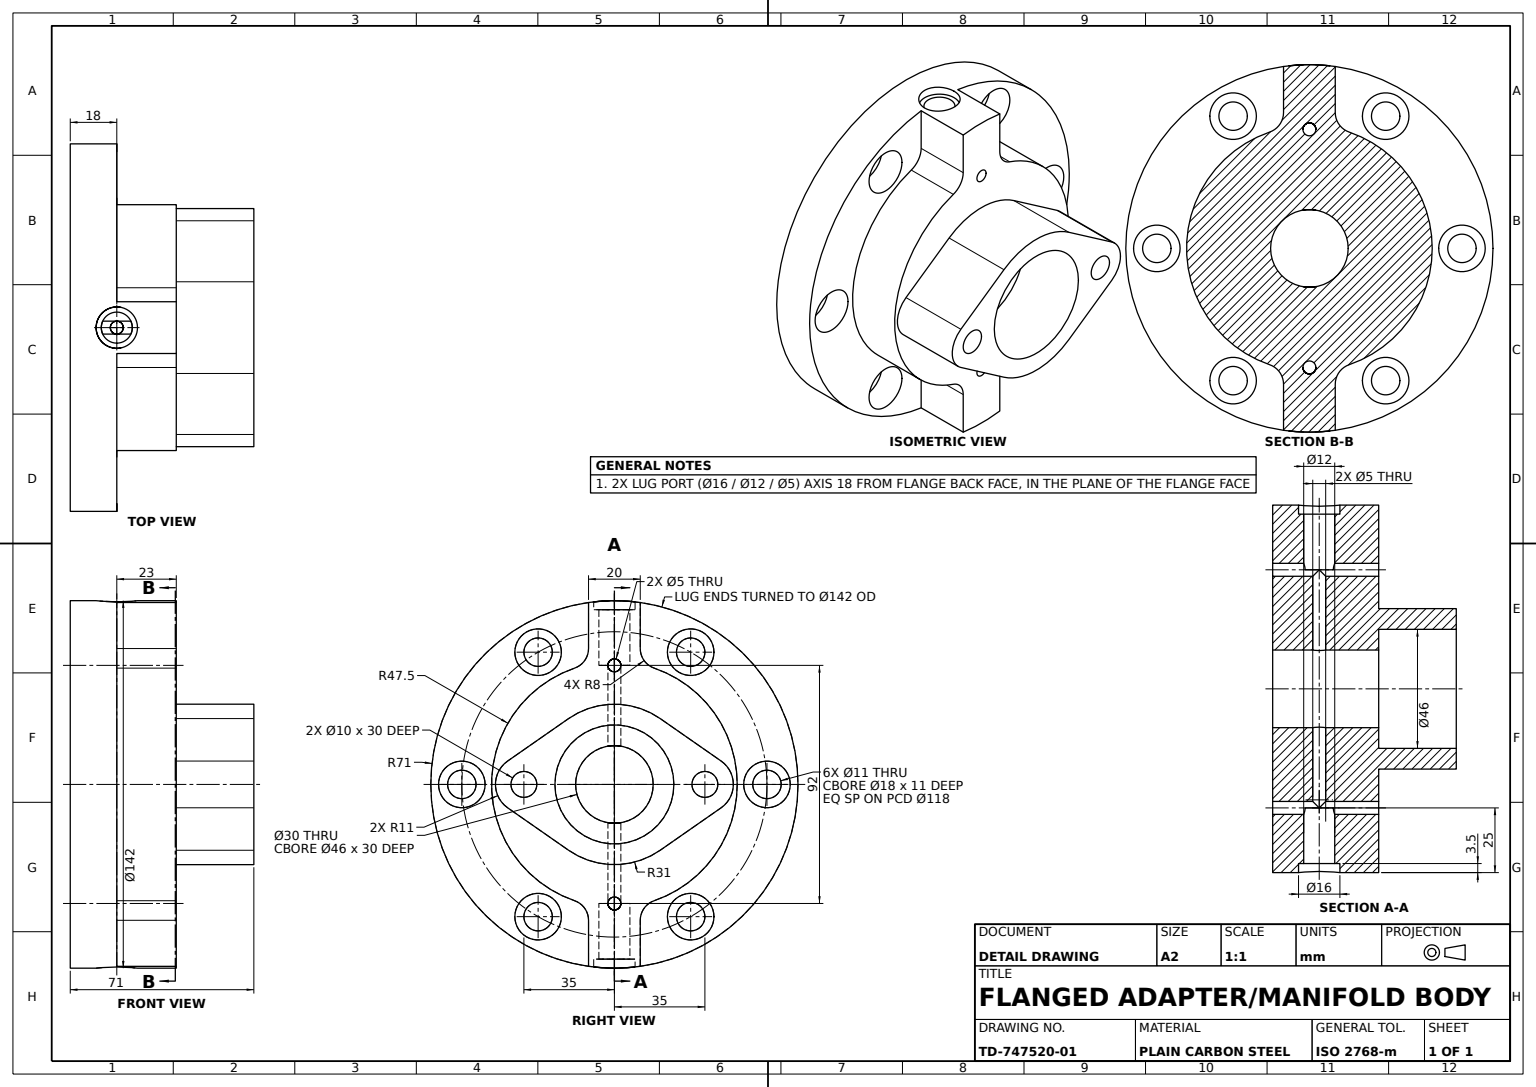
from build123d import *
from build123d.topology import SkipClean

# Parameters (mm, degrees)
BASE_FLANGE_SKETCH_R            = 71
BASE_FLANGE_SKETCH_R_2          = 5.5
BASE_FLANGE_142_6X_11_DEPTH     = 18
FLANGE_COUNTERBORE_SKETCH_R     = 9
FLANGE_COUNTERBORES_6X_18_DEPTH = 11
HUB_95_WITH_SIDE_LUGS_DEPTH     = 23
LOBED_CAP_SKETCH_R              = 5
LOBED_CAP_SKETCH_R_2            = 23
LOBED_CAP_BOSS_DEPTH            = 30
CAP_HOLES_SKETCH_R              = 2.5
CAP_HOLES_2X_5_DEPTH            = 60
BORE_SKETCH_R                   = 15
BORE_30_DEPTH                   = 71
CROSS_HOLE_SKETCH_R             = 2.5
CROSS_HOLE_5_DEPTH              = 200
SIDE_A_COUNTERBORE_SKETCH_R     = 6
SIDE_A_COUNTERBORE_12_DEPTH     = 25
SIDE_A_SPOTFACE_SKETCH_R        = 8
SIDE_A_SPOTFACE_16_DEPTH        = 3.5
SIDE_START                      = 25
SIDE_B_COUNTERBORE_SKETCH_R     = 6
SIDE_B_COUNTERBORE_12_DEPTH     = 25
SIDE_START_2                    = 3.5
SIDE_B_SPOTFACE_SKETCH_R        = 8
SIDE_B_SPOTFACE_16_DEPTH        = 3.5


with BuildPart() as part:
    # Base Flange Sketch → Base Flange Ø142 6xØ11 (new body)
    with BuildSketch(Plane(origin=(0, 0, 0), x_dir=(1, 0, 0), z_dir=(0, 1, 0))):
        with Locations(Location((0, 0, 0), (0, 0, 270))):
            Circle(BASE_FLANGE_SKETCH_R)
        with Locations(Location((0, 59, 0), (0, 0, 270))):
            Circle(BASE_FLANGE_SKETCH_R_2, mode=Mode.SUBTRACT)
        with Locations(Location((51.095498823, 29.5, 0), (0, 0, 270))):
            Circle(BASE_FLANGE_SKETCH_R_2, mode=Mode.SUBTRACT)
        with Locations(Location((51.095498823, -29.5, 0), (0, 0, 270))):
            Circle(BASE_FLANGE_SKETCH_R_2, mode=Mode.SUBTRACT)
        with Locations(Location((0, -59, 0), (0, 0, 270))):
            Circle(BASE_FLANGE_SKETCH_R_2, mode=Mode.SUBTRACT)
        with Locations(Location((-51.095498823, -29.5, 0), (0, 0, 270))):
            Circle(BASE_FLANGE_SKETCH_R_2, mode=Mode.SUBTRACT)
        with Locations(Location((-51.095498823, 29.5, 0), (0, 0, 270))):
            Circle(BASE_FLANGE_SKETCH_R_2, mode=Mode.SUBTRACT)
    extrude(amount=BASE_FLANGE_142_6X_11_DEPTH)

    # Flange Counterbore Sketch → Flange Counterbores 6xØ18 (cut)
    with BuildSketch(Plane(origin=(0, 18, 0), x_dir=(1, 0, 0), z_dir=(0, 1, 0))):
        with Locations(Location((0, 59, 0), (0, 0, 270))):
            Circle(FLANGE_COUNTERBORE_SKETCH_R)
        with Locations(Location((51.095498823, 29.5, 0), (0, 0, 270))):
            Circle(FLANGE_COUNTERBORE_SKETCH_R)
        with Locations(Location((51.095498823, -29.5, 0), (0, 0, 270))):
            Circle(FLANGE_COUNTERBORE_SKETCH_R)
        with Locations(Location((0, -59, 0), (0, 0, 270))):
            Circle(FLANGE_COUNTERBORE_SKETCH_R)
        with Locations(Location((-51.095498823, -29.5, 0), (0, 0, 270))):
            Circle(FLANGE_COUNTERBORE_SKETCH_R)
        with Locations(Location((-51.095498823, 29.5, 0), (0, 0, 270))):
            Circle(FLANGE_COUNTERBORE_SKETCH_R)
    extrude(amount=-FLANGE_COUNTERBORES_6X_18_DEPTH, mode=Mode.SUBTRACT)

    # Hub Sketch → Hub Ø95 with Side Lugs (add)
    with SkipClean():  # the faces are left unmerged after this step: merging them gives an invalid solid
        with BuildSketch(Plane(origin=(0, 18, 0), x_dir=(1, 0, 0), z_dir=(0, 1, 0))):
            with BuildLine():
                Line((52.5, 10), (70.292247083, 10))
                ThreePointArc((70.292247083, 10), (71, 0), (70.292247083, -10))
                Line((70.292247083, -10), (52.5, -10))
                ThreePointArc((52.5, -10), (47.85009445, -11.49013223), (44.932432432, -15.405405405))
                ThreePointArc((44.932432432, -15.405405405), (0, -47.5), (-44.932432432, -15.405405405))
                ThreePointArc((-44.932432432, -15.405405405), (-47.85009445, -11.49013223), (-52.5, -10))
                Line((-52.5, -10), (-70.292247083, -10))
                ThreePointArc((-70.292247083, -10), (-71, 0), (-70.292247083, 10))
                Line((-70.292247083, 10), (-52.5, 10))
                ThreePointArc((-52.5, 10), (-47.85009445, 11.49013223), (-44.932432432, 15.405405405))
                ThreePointArc((-44.932432432, 15.405405405), (0, 47.5), (44.932432432, 15.405405405))
                ThreePointArc((44.932432432, 15.405405405), (47.85009445, 11.49013223), (52.5, 10))
            make_face()
        extrude(amount=HUB_95_WITH_SIDE_LUGS_DEPTH)

    # Lobed Cap Sketch → Lobed Cap Boss (add)
    with SkipClean():  # the faces are left unmerged after this step: merging them gives an invalid solid
        with BuildSketch(Plane(origin=(0, 41, 0), x_dir=(1, 0, 0), z_dir=(0, 1, 0))):
            with BuildLine():
                Line((-25.440206006, 17.714285714), (-9.027169873, 41.285714286))
                ThreePointArc((-9.027169873, 41.285714286), (0, 46), (9.027169873, 41.285714286))
                Line((9.027169873, 41.285714286), (25.440206006, 17.714285714))
                ThreePointArc((25.440206006, 17.714285714), (31, 0), (25.440206006, -17.714285714))
                Line((25.440206006, -17.714285714), (9.027169873, -41.285714286))
                ThreePointArc((9.027169873, -41.285714286), (0, -46), (-9.027169873, -41.285714286))
                Line((-9.027169873, -41.285714286), (-25.440206006, -17.714285714))
                ThreePointArc((-25.440206006, -17.714285714), (-31, 0), (-25.440206006, 17.714285714))
            make_face()
            with Locations(Location((0, 35, 0), (0, 0, 270))):
                Circle(LOBED_CAP_SKETCH_R, mode=Mode.SUBTRACT)
            with Locations(Location((0, -35, 0), (0, 0, 270))):
                Circle(LOBED_CAP_SKETCH_R, mode=Mode.SUBTRACT)
            with Locations(Location((0, 0, 0), (0, 0, 270))):
                Circle(LOBED_CAP_SKETCH_R_2, mode=Mode.SUBTRACT)
        extrude(amount=LOBED_CAP_BOSS_DEPTH)

    # Cap Holes Sketch → Cap Holes 2xØ5 (cut)
    with SkipClean():  # the faces are left unmerged after this step: merging them gives an invalid solid
        with BuildSketch(Plane(origin=(0, 41, 0), x_dir=(1, 0, 0), z_dir=(0, 1, 0))):
            with Locations(Location((-46, 0, 0), (0, 0, 270))):
                Circle(CAP_HOLES_SKETCH_R)
            with Locations(Location((46, 0, 0), (0, 0, 270))):
                Circle(CAP_HOLES_SKETCH_R)
        extrude(amount=-CAP_HOLES_2X_5_DEPTH, mode=Mode.SUBTRACT)

    # Bore Sketch → Bore Ø30 (cut)
    with SkipClean():  # the faces are left unmerged after this step: merging them gives an invalid solid
        with BuildSketch(Plane(origin=(0, 71, 0), x_dir=(1, 0, 0), z_dir=(0, 1, 0))):
            with Locations(Location((0, 0, 0), (0, 0, 270))):
                Circle(BORE_SKETCH_R)
        extrude(amount=-BORE_30_DEPTH, mode=Mode.SUBTRACT)

    # Cross Hole Sketch → Cross Hole Ø5 (cut)
    with BuildSketch(Plane(origin=(71, 0, 0), x_dir=(0, 0, -1), z_dir=(1, 0, 0))):
        with Locations((0, 18)):
            Circle(CROSS_HOLE_SKETCH_R)
    extrude(amount=-CROSS_HOLE_5_DEPTH, mode=Mode.SUBTRACT)

    # Side A Counterbore Sketch → Side A Counterbore Ø12 (cut)
    with BuildSketch(Plane(origin=(71, 0, 0), x_dir=(0, 0, -1), z_dir=(1, 0, 0))):
        with Locations((0, 18)):
            Circle(SIDE_A_COUNTERBORE_SKETCH_R)
    extrude(amount=-SIDE_A_COUNTERBORE_12_DEPTH, mode=Mode.SUBTRACT)

    # Side A Spotface Sketch → Side A Spotface Ø16 (cut)
    with BuildSketch(Plane(origin=(71, 0, 0), x_dir=(0, 0, -1), z_dir=(1, 0, 0))):
        with Locations((0, 18)):
            Circle(SIDE_A_SPOTFACE_SKETCH_R)
    extrude(amount=-SIDE_A_SPOTFACE_16_DEPTH, mode=Mode.SUBTRACT)

    # Side B Counterbore Sketch → Side B Counterbore Ø12 (cut)
    with BuildSketch(Plane(origin=(-71, 0, 0), x_dir=(0, 0, -1), z_dir=(1, 0, 0)).offset(SIDE_START)):
        with Locations((0, 18)):
            Circle(SIDE_B_COUNTERBORE_SKETCH_R)
    extrude(amount=-SIDE_B_COUNTERBORE_12_DEPTH, mode=Mode.SUBTRACT)

    # Side B Spotface Sketch → Side B Spotface Ø16 (cut)
    with BuildSketch(Plane(origin=(-71, 0, 0), x_dir=(0, 0, -1), z_dir=(1, 0, 0)).offset(SIDE_START_2)):
        with Locations((0, 18)):
            Circle(SIDE_B_SPOTFACE_SKETCH_R)
    extrude(amount=-SIDE_B_SPOTFACE_16_DEPTH, mode=Mode.SUBTRACT)


solid = part.part
